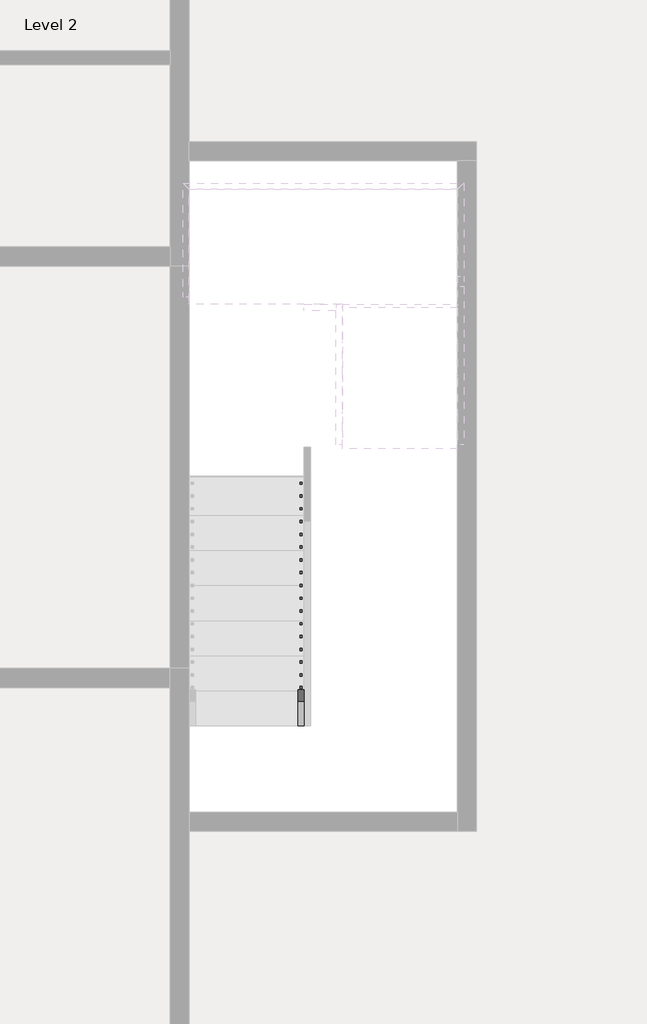
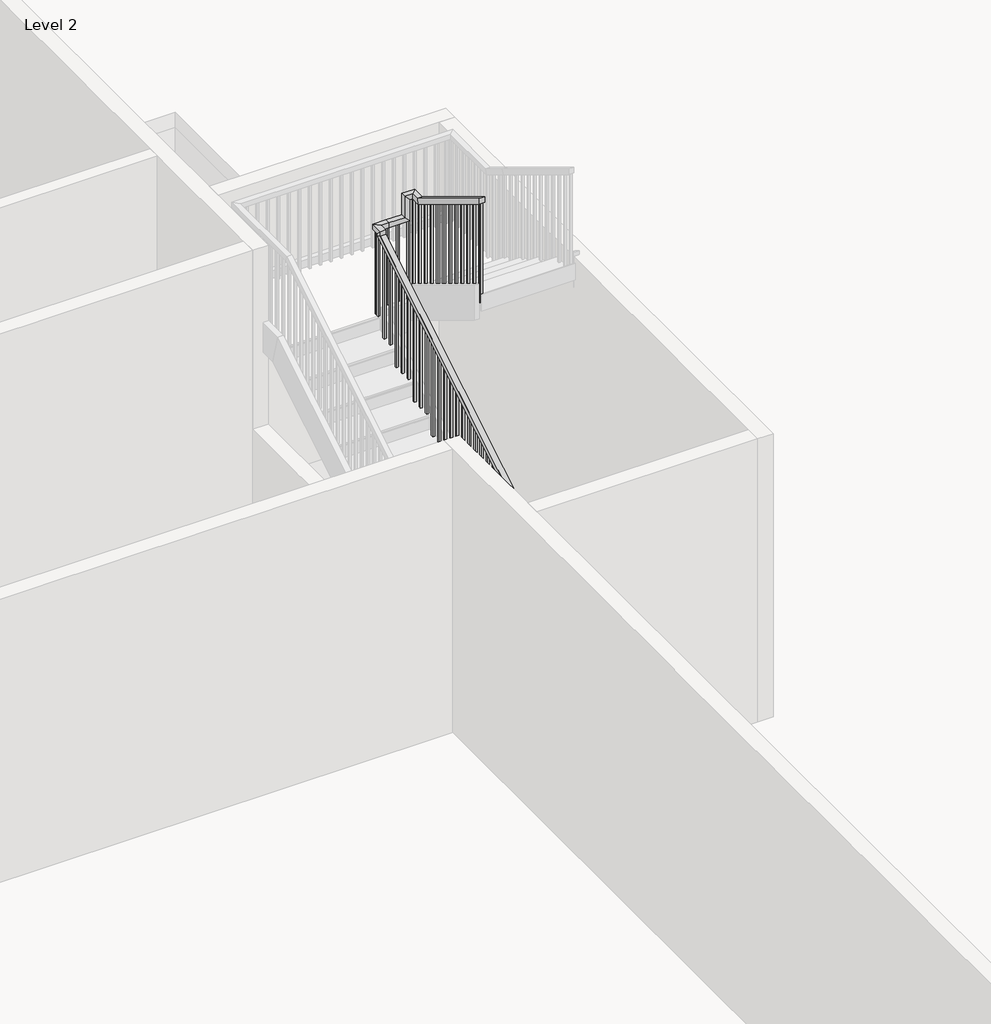
# One storey, part 7 of 8: 1 railing.
"""IFC4 building model written with IfcOpenShell, lengths in millimetres."""

from ifc_helpers import new_model, si_unit, frame, origin, place, context, project, spatial, polyline, outline, extrude, faceted_brep, element, save

model = new_model("IFC4")

# Units and contexts
model_context = context("Model", 3, world=origin())
ifc_project = project(units=[si_unit("LENGTHUNIT", "METRE", prefix="MILLI")], contexts=[model_context])

# Site, building, storey
site = spatial("IfcSite", under=ifc_project)
building = spatial("IfcBuilding", under=site)
storey = spatial("IfcBuildingStorey", under=building, Name="Level 2", Elevation=28282.6172466)

# Railing
placement = place(None, origin())
element("IfcRailing", 1, ObjectType="Handrail - Rectangular", at=placement, inside=storey, context=model_context, shape_type="SolidModel", body=[
    faceted_brep([(-2753.8415084, 19841.9216096, 29366.3505799), (-2753.8415084, 19841.9216096, 29306.9491197), (-2703.0415084, 19841.9216096, 29306.9491197), (-2703.0415084, 19841.9216096, 29366.3505799), (-2753.8415084, 23118.5216096, 31352.1687618), (-2753.8415084, 23169.3216096, 31323.5551803), (-2703.0415084, 23169.3216096, 31323.5551803), (-2703.0415084, 23118.5216096, 31352.1687618), (-2753.8415084, 23118.5216096, 31398.3505799), (-2753.8415084, 23169.3216096, 31347.5505799), (-2703.0415084, 23169.3216096, 31347.5505799), (-2703.0415084, 23118.5216096, 31398.3505799), (-2753.8415084, 23245.5216096, 31398.3505799), (-2753.8415084, 23245.5216096, 31347.5505799), (-2703.0415084, 23194.7216096, 31347.5505799), (-2703.0415084, 23194.7216096, 31398.3505799), (-2626.8415084, 23245.5216096, 31398.3505799), (-2626.8415084, 23245.5216096, 31347.5505799), (-2626.8415084, 23194.7216096, 31347.5505799), (-2626.8415084, 23194.7216096, 31398.3505799), (-2474.4415084, 23245.5216096, 31398.3505799), (-2423.6415084, 23245.5216096, 31347.5505799), (-2423.6415084, 23194.7216096, 31347.5505799), (-2474.4415084, 23194.7216096, 31398.3505799), (-2474.4415084, 23245.5216096, 31613.8657314), (-2423.6415084, 23245.5216096, 31563.0657314), (-2423.6415084, 23194.7216096, 31563.0657314), (-2474.4415084, 23194.7216096, 31613.8657314), (-2347.4415084, 23245.5216096, 31613.8657314), (-2347.4415084, 23245.5216096, 31563.0657314), (-2398.2415084, 23194.7216096, 31563.0657314), (-2398.2415084, 23194.7216096, 31613.8657314), (-2347.4415084, 23118.5216096, 31613.8657314), (-2347.4415084, 23104.3292002, 31563.0657314), (-2398.2415084, 23104.3292002, 31563.0657314), (-2398.2415084, 23118.5216096, 31613.8657314), (-2347.4415084, 22077.1216096, 32245.0172466), (-2398.2415084, 22077.1216096, 32245.0172466), (-2398.2415084, 22077.1216096, 32185.6157863), (-2347.4415084, 22077.1216096, 32185.6157863)], [[[0, 1, 2, 3]], [[1, 0, 4, 5]], [[2, 1, 5, 6]], [[3, 2, 6, 7]], [[0, 3, 7, 4]], [[5, 4, 8, 9]], [[6, 5, 9, 10]], [[7, 6, 10, 11]], [[4, 7, 11, 8]], [[9, 8, 12, 13]], [[10, 9, 13, 14]], [[11, 10, 14, 15]], [[8, 11, 15, 12]], [[13, 12, 16, 17]], [[14, 13, 17, 18]], [[15, 14, 18, 19]], [[12, 15, 19, 16]], [[17, 16, 20, 21]], [[18, 17, 21, 22]], [[19, 18, 22, 23]], [[16, 19, 23, 20]], [[21, 20, 24, 25]], [[22, 21, 25, 26]], [[23, 22, 26, 27]], [[20, 23, 27, 24]], [[25, 24, 28, 29]], [[26, 25, 29, 30]], [[27, 26, 30, 31]], [[24, 27, 31, 28]], [[29, 28, 32, 33]], [[30, 29, 33, 34]], [[31, 30, 34, 35]], [[28, 31, 35, 32]], [[36, 37, 38, 39]], [[33, 32, 36, 39]], [[34, 33, 39, 38]], [[35, 34, 38, 37]], [[32, 35, 37, 36]]]),
    extrude(outline(polyline([(22092.9966096, 32175.9945742), (22112.0466096, 32164.4491197), (22112.0466096, 31161.2839133), (22092.9966096, 31161.2839133), (22092.9966096, 32175.9945742)])), frame((-2382.3665084, 0.0, 0.0), z_axis=(1.0, 0.0, 0.0), x_axis=(0.0, 1.0, 0.0)), (0.0, 0.0, 1.0), 19.05),
    extrude(outline(polyline([(22194.5966096, 32114.4188166), (22213.6466096, 32102.8733621), (22213.6466096, 31161.2839133), (22194.5966096, 31161.2839133), (22194.5966096, 32114.4188166)])), frame((-2382.3665084, 0.0, 0.0), z_axis=(1.0, 0.0, 0.0), x_axis=(0.0, 1.0, 0.0)), (0.0, 0.0, 1.0), 19.05),
    extrude(outline(polyline([(22296.1966096, 32052.8430591), (22315.2466096, 32041.2976045), (22315.2466096, 31161.2839133), (22296.1966096, 31161.2839133), (22296.1966096, 32052.8430591)])), frame((-2382.3665084, 0.0, 0.0), z_axis=(1.0, 0.0, 0.0), x_axis=(0.0, 1.0, 0.0)), (0.0, 0.0, 1.0), 19.05),
    extrude(outline(polyline([(22397.7966096, 31991.2673015), (22416.8466096, 31979.721847), (22416.8466096, 30991.9505799), (22397.7966096, 30991.9505799), (22397.7966096, 31991.2673015)])), frame((-2382.3665084, 0.0, 0.0), z_axis=(1.0, 0.0, 0.0), x_axis=(0.0, 1.0, 0.0)), (0.0, 0.0, 1.0), 19.05),
    extrude(outline(polyline([(22499.3966096, 31929.6915439), (22518.4466096, 31918.1460894), (22518.4466096, 30991.9505799), (22499.3966096, 30991.9505799), (22499.3966096, 31929.6915439)])), frame((-2382.3665084, 0.0, 0.0), z_axis=(1.0, 0.0, 0.0), x_axis=(0.0, 1.0, 0.0)), (0.0, 0.0, 1.0), 19.05),
    extrude(outline(polyline([(22600.9966096, 31868.1157863), (22620.0466096, 31856.5703318), (22620.0466096, 30991.9505799), (22600.9966096, 30991.9505799), (22600.9966096, 31868.1157863)])), frame((-2382.3665084, 0.0, 0.0), z_axis=(1.0, 0.0, 0.0), x_axis=(0.0, 1.0, 0.0)), (0.0, 0.0, 1.0), 19.05),
    extrude(outline(polyline([(22702.5966096, 31806.5400288), (22721.6466096, 31794.9945742), (22721.6466096, 30822.6172466), (22702.5966096, 30822.6172466), (22702.5966096, 31806.5400288)])), frame((-2382.3665084, 0.0, 0.0), z_axis=(1.0, 0.0, 0.0), x_axis=(0.0, 1.0, 0.0)), (0.0, 0.0, 1.0), 19.05),
    extrude(outline(polyline([(22804.1966096, 31744.9642712), (22823.2466096, 31733.4188166), (22823.2466096, 30822.6172466), (22804.1966096, 30822.6172466), (22804.1966096, 31744.9642712)])), frame((-2382.3665084, 0.0, 0.0), z_axis=(1.0, 0.0, 0.0), x_axis=(0.0, 1.0, 0.0)), (0.0, 0.0, 1.0), 19.05),
    extrude(outline(polyline([(22905.7966096, 31683.3885136), (22924.8466096, 31671.8430591), (22924.8466096, 30822.6172466), (22905.7966096, 30822.6172466), (22905.7966096, 31683.3885136)])), frame((-2382.3665084, 0.0, 0.0), z_axis=(1.0, 0.0, 0.0), x_axis=(0.0, 1.0, 0.0)), (0.0, 0.0, 1.0), 19.05),
    extrude(outline(polyline([(23007.3966096, 31621.812756), (23026.4466096, 31610.2673015), (23026.4466096, 30653.2839133), (23007.3966096, 30653.2839133), (23007.3966096, 31621.812756)])), frame((-2382.3665084, 0.0, 0.0), z_axis=(1.0, 0.0, 0.0), x_axis=(0.0, 1.0, 0.0)), (0.0, 0.0, 1.0), 19.05),
    extrude(outline(polyline([(23108.9966096, 31560.2369985), (23128.0466096, 31548.6915439), (23128.0466096, 30653.2839133), (23108.9966096, 30653.2839133), (23108.9966096, 31560.2369985)])), frame((-2382.3665084, 0.0, 0.0), z_axis=(1.0, 0.0, 0.0), x_axis=(0.0, 1.0, 0.0)), (0.0, 0.0, 1.0), 19.05),
    extrude(outline(polyline([(-2433.1665084, 23210.5966096), (-2433.1665084, 23229.6466096), (-2414.1165084, 23229.6466096), (-2414.1165084, 23210.5966096), (-2433.1665084, 23210.5966096)])), frame((0.0, 0.0, 30483.9505799), z_axis=(0.0, 0.0, 1.0), x_axis=(1.0, 0.0, 0.0)), (0.0, 0.0, 1.0), 1079.1151515),
    extrude(outline(polyline([(-2534.7665084, 23210.5966096), (-2534.7665084, 23229.6466096), (-2515.7165084, 23229.6466096), (-2515.7165084, 23210.5966096), (-2534.7665084, 23210.5966096)])), frame((0.0, 0.0, 30483.9505799), z_axis=(0.0, 0.0, 1.0), x_axis=(1.0, 0.0, 0.0)), (0.0, 0.0, 1.0), 863.6),
    extrude(outline(polyline([(-2636.3665084, 23210.5966096), (-2636.3665084, 23229.6466096), (-2617.3165084, 23229.6466096), (-2617.3165084, 23210.5966096), (-2636.3665084, 23210.5966096)])), frame((0.0, 0.0, 30483.9505799), z_axis=(0.0, 0.0, 1.0), x_axis=(1.0, 0.0, 0.0)), (0.0, 0.0, 1.0), 863.6),
    extrude(outline(polyline([(-2718.9165084, 23185.1966096), (-2737.9665084, 23185.1966096), (-2737.9665084, 23204.2466096), (-2718.9165084, 23204.2466096), (-2718.9165084, 23185.1966096)])), frame((0.0, 0.0, 30483.9505799), z_axis=(0.0, 0.0, 1.0), x_axis=(1.0, 0.0, 0.0)), (0.0, 0.0, 1.0), 863.6),
    extrude(outline(polyline([(23083.5966096, 31271.6006348), (23102.6466096, 31283.1460894), (23102.6466096, 30314.6172466), (23083.5966096, 30314.6172466), (23083.5966096, 31271.6006348)])), frame((-2737.9665084, 0.0, 0.0), z_axis=(1.0, 0.0, 0.0), x_axis=(0.0, 1.0, 0.0)), (0.0, 0.0, 1.0), 19.05),
    extrude(outline(polyline([(22981.9966096, 31210.0248773), (23001.0466096, 31221.5703318), (23001.0466096, 30314.6172466), (22981.9966096, 30314.6172466), (22981.9966096, 31210.0248773)])), frame((-2737.9665084, 0.0, 0.0), z_axis=(1.0, 0.0, 0.0), x_axis=(0.0, 1.0, 0.0)), (0.0, 0.0, 1.0), 19.05),
    extrude(outline(polyline([(22880.3966096, 31148.4491197), (22899.4466096, 31159.9945742), (22899.4466096, 30145.2839133), (22880.3966096, 30145.2839133), (22880.3966096, 31148.4491197)])), frame((-2737.9665084, 0.0, 0.0), z_axis=(1.0, 0.0, 0.0), x_axis=(0.0, 1.0, 0.0)), (0.0, 0.0, 1.0), 19.05),
    extrude(outline(polyline([(22778.7966096, 31086.8733621), (22797.8466096, 31098.4188167), (22797.8466096, 30145.2839133), (22778.7966096, 30145.2839133), (22778.7966096, 31086.8733621)])), frame((-2737.9665084, 0.0, 0.0), z_axis=(1.0, 0.0, 0.0), x_axis=(0.0, 1.0, 0.0)), (0.0, 0.0, 1.0), 19.05),
    extrude(outline(polyline([(22677.1966096, 31025.2976045), (22696.2466096, 31036.8430591), (22696.2466096, 30145.2839133), (22677.1966096, 30145.2839133), (22677.1966096, 31025.2976045)])), frame((-2737.9665084, 0.0, 0.0), z_axis=(1.0, 0.0, 0.0), x_axis=(0.0, 1.0, 0.0)), (0.0, 0.0, 1.0), 19.05),
    extrude(outline(polyline([(22575.5966096, 30963.721847), (22594.6466096, 30975.2673015), (22594.6466096, 29975.9505799), (22575.5966096, 29975.9505799), (22575.5966096, 30963.721847)])), frame((-2737.9665084, 0.0, 0.0), z_axis=(1.0, 0.0, 0.0), x_axis=(0.0, 1.0, 0.0)), (0.0, 0.0, 1.0), 19.05),
    extrude(outline(polyline([(22473.9966096, 30902.1460894), (22493.0466096, 30913.6915439), (22493.0466096, 29975.9505799), (22473.9966096, 29975.9505799), (22473.9966096, 30902.1460894)])), frame((-2737.9665084, 0.0, 0.0), z_axis=(1.0, 0.0, 0.0), x_axis=(0.0, 1.0, 0.0)), (0.0, 0.0, 1.0), 19.05),
    extrude(outline(polyline([(22372.3966096, 30840.5703318), (22391.4466096, 30852.1157863), (22391.4466096, 29975.9505799), (22372.3966096, 29975.9505799), (22372.3966096, 30840.5703318)])), frame((-2737.9665084, 0.0, 0.0), z_axis=(1.0, 0.0, 0.0), x_axis=(0.0, 1.0, 0.0)), (0.0, 0.0, 1.0), 19.05),
    extrude(outline(polyline([(22270.7966096, 30778.9945742), (22289.8466096, 30790.5400288), (22289.8466096, 29806.6172466), (22270.7966096, 29806.6172466), (22270.7966096, 30778.9945742)])), frame((-2737.9665084, 0.0, 0.0), z_axis=(1.0, 0.0, 0.0), x_axis=(0.0, 1.0, 0.0)), (0.0, 0.0, 1.0), 19.05),
    extrude(outline(polyline([(22169.1966096, 30717.4188167), (22188.2466096, 30728.9642712), (22188.2466096, 29806.6172466), (22169.1966096, 29806.6172466), (22169.1966096, 30717.4188167)])), frame((-2737.9665084, 0.0, 0.0), z_axis=(1.0, 0.0, 0.0), x_axis=(0.0, 1.0, 0.0)), (0.0, 0.0, 1.0), 19.05),
    extrude(outline(polyline([(22067.5966096, 30655.8430591), (22086.6466096, 30667.3885136), (22086.6466096, 29806.6172466), (22067.5966096, 29806.6172466), (22067.5966096, 30655.8430591)])), frame((-2737.9665084, 0.0, 0.0), z_axis=(1.0, 0.0, 0.0), x_axis=(0.0, 1.0, 0.0)), (0.0, 0.0, 1.0), 19.05),
    extrude(outline(polyline([(21965.9966096, 30594.2673015), (21985.0466096, 30605.812756), (21985.0466096, 29637.2839133), (21965.9966096, 29637.2839133), (21965.9966096, 30594.2673015)])), frame((-2737.9665084, 0.0, 0.0), z_axis=(1.0, 0.0, 0.0), x_axis=(0.0, 1.0, 0.0)), (0.0, 0.0, 1.0), 19.05),
    extrude(outline(polyline([(21864.3966096, 30532.6915439), (21883.4466096, 30544.2369985), (21883.4466096, 29637.2839133), (21864.3966096, 29637.2839133), (21864.3966096, 30532.6915439)])), frame((-2737.9665084, 0.0, 0.0), z_axis=(1.0, 0.0, 0.0), x_axis=(0.0, 1.0, 0.0)), (0.0, 0.0, 1.0), 19.05),
    extrude(outline(polyline([(21762.7966096, 30471.1157863), (21781.8466096, 30482.6612409), (21781.8466096, 29467.9505799), (21762.7966096, 29467.9505799), (21762.7966096, 30471.1157863)])), frame((-2737.9665084, 0.0, 0.0), z_axis=(1.0, 0.0, 0.0), x_axis=(0.0, 1.0, 0.0)), (0.0, 0.0, 1.0), 19.05),
    extrude(outline(polyline([(21661.1966096, 30409.5400288), (21680.2466096, 30421.0854833), (21680.2466096, 29467.9505799), (21661.1966096, 29467.9505799), (21661.1966096, 30409.5400288)])), frame((-2737.9665084, 0.0, 0.0), z_axis=(1.0, 0.0, 0.0), x_axis=(0.0, 1.0, 0.0)), (0.0, 0.0, 1.0), 19.05),
    extrude(outline(polyline([(21559.5966096, 30347.9642712), (21578.6466096, 30359.5097257), (21578.6466096, 29467.9505799), (21559.5966096, 29467.9505799), (21559.5966096, 30347.9642712)])), frame((-2737.9665084, 0.0, 0.0), z_axis=(1.0, 0.0, 0.0), x_axis=(0.0, 1.0, 0.0)), (0.0, 0.0, 1.0), 19.05),
    extrude(outline(polyline([(21457.9966096, 30286.3885136), (21477.0466096, 30297.9339682), (21477.0466096, 29298.6172466), (21457.9966096, 29298.6172466), (21457.9966096, 30286.3885136)])), frame((-2737.9665084, 0.0, 0.0), z_axis=(1.0, 0.0, 0.0), x_axis=(0.0, 1.0, 0.0)), (0.0, 0.0, 1.0), 19.05),
    extrude(outline(polyline([(21356.3966096, 30224.812756), (21375.4466096, 30236.3582106), (21375.4466096, 29298.6172466), (21356.3966096, 29298.6172466), (21356.3966096, 30224.812756)])), frame((-2737.9665084, 0.0, 0.0), z_axis=(1.0, 0.0, 0.0), x_axis=(0.0, 1.0, 0.0)), (0.0, 0.0, 1.0), 19.05),
    extrude(outline(polyline([(21254.7966096, 30163.2369985), (21273.8466096, 30174.782453), (21273.8466096, 29298.6172466), (21254.7966096, 29298.6172466), (21254.7966096, 30163.2369985)])), frame((-2737.9665084, 0.0, 0.0), z_axis=(1.0, 0.0, 0.0), x_axis=(0.0, 1.0, 0.0)), (0.0, 0.0, 1.0), 19.05),
    extrude(outline(polyline([(21153.1966096, 30101.6612409), (21172.2466096, 30113.2066954), (21172.2466096, 29129.2839133), (21153.1966096, 29129.2839133), (21153.1966096, 30101.6612409)])), frame((-2737.9665084, 0.0, 0.0), z_axis=(1.0, 0.0, 0.0), x_axis=(0.0, 1.0, 0.0)), (0.0, 0.0, 1.0), 19.05),
    extrude(outline(polyline([(21051.5966096, 30040.0854833), (21070.6466096, 30051.6309379), (21070.6466096, 29129.2839133), (21051.5966096, 29129.2839133), (21051.5966096, 30040.0854833)])), frame((-2737.9665084, 0.0, 0.0), z_axis=(1.0, 0.0, 0.0), x_axis=(0.0, 1.0, 0.0)), (0.0, 0.0, 1.0), 19.05),
    extrude(outline(polyline([(20949.9966096, 29978.5097257), (20969.0466096, 29990.0551803), (20969.0466096, 29129.2839133), (20949.9966096, 29129.2839133), (20949.9966096, 29978.5097257)])), frame((-2737.9665084, 0.0, 0.0), z_axis=(1.0, 0.0, 0.0), x_axis=(0.0, 1.0, 0.0)), (0.0, 0.0, 1.0), 19.05),
    extrude(outline(polyline([(20848.3966096, 29916.9339682), (20867.4466096, 29928.4794227), (20867.4466096, 28959.9505799), (20848.3966096, 28959.9505799), (20848.3966096, 29916.9339682)])), frame((-2737.9665084, 0.0, 0.0), z_axis=(1.0, 0.0, 0.0), x_axis=(0.0, 1.0, 0.0)), (0.0, 0.0, 1.0), 19.05),
    extrude(outline(polyline([(20746.7966096, 29855.3582106), (20765.8466096, 29866.9036651), (20765.8466096, 28959.9505799), (20746.7966096, 28959.9505799), (20746.7966096, 29855.3582106)])), frame((-2737.9665084, 0.0, 0.0), z_axis=(1.0, 0.0, 0.0), x_axis=(0.0, 1.0, 0.0)), (0.0, 0.0, 1.0), 19.05),
    extrude(outline(polyline([(20645.1966096, 29793.782453), (20664.2466096, 29805.3279076), (20664.2466096, 28790.6172466), (20645.1966096, 28790.6172466), (20645.1966096, 29793.782453)])), frame((-2737.9665084, 0.0, 0.0), z_axis=(1.0, 0.0, 0.0), x_axis=(0.0, 1.0, 0.0)), (0.0, 0.0, 1.0), 19.05),
    extrude(outline(polyline([(20543.5966096, 29732.2066954), (20562.6466096, 29743.75215), (20562.6466096, 28790.6172466), (20543.5966096, 28790.6172466), (20543.5966096, 29732.2066954)])), frame((-2737.9665084, 0.0, 0.0), z_axis=(1.0, 0.0, 0.0), x_axis=(0.0, 1.0, 0.0)), (0.0, 0.0, 1.0), 19.05),
    extrude(outline(polyline([(20441.9966096, 29670.6309379), (20461.0466096, 29682.1763924), (20461.0466096, 28790.6172466), (20441.9966096, 28790.6172466), (20441.9966096, 29670.6309379)])), frame((-2737.9665084, 0.0, 0.0), z_axis=(1.0, 0.0, 0.0), x_axis=(0.0, 1.0, 0.0)), (0.0, 0.0, 1.0), 19.05),
    extrude(outline(polyline([(20340.3966096, 29609.0551803), (20359.4466096, 29620.6006348), (20359.4466096, 28621.2839133), (20340.3966096, 28621.2839133), (20340.3966096, 29609.0551803)])), frame((-2737.9665084, 0.0, 0.0), z_axis=(1.0, 0.0, 0.0), x_axis=(0.0, 1.0, 0.0)), (0.0, 0.0, 1.0), 19.05),
    extrude(outline(polyline([(20238.7966096, 29547.4794227), (20257.8466096, 29559.0248773), (20257.8466096, 28621.2839133), (20238.7966096, 28621.2839133), (20238.7966096, 29547.4794227)])), frame((-2737.9665084, 0.0, 0.0), z_axis=(1.0, 0.0, 0.0), x_axis=(0.0, 1.0, 0.0)), (0.0, 0.0, 1.0), 19.05),
    extrude(outline(polyline([(20137.1966096, 29485.9036651), (20156.2466096, 29497.4491197), (20156.2466096, 28621.2839133), (20137.1966096, 28621.2839133), (20137.1966096, 29485.9036651)])), frame((-2737.9665084, 0.0, 0.0), z_axis=(1.0, 0.0, 0.0), x_axis=(0.0, 1.0, 0.0)), (0.0, 0.0, 1.0), 19.05),
    extrude(outline(polyline([(20035.5966096, 29424.3279076), (20054.6466096, 29435.8733621), (20054.6466096, 28451.9505799), (20035.5966096, 28451.9505799), (20035.5966096, 29424.3279076)])), frame((-2737.9665084, 0.0, 0.0), z_axis=(1.0, 0.0, 0.0), x_axis=(0.0, 1.0, 0.0)), (0.0, 0.0, 1.0), 19.05),
    extrude(outline(polyline([(19933.9966096, 29362.75215), (19953.0466096, 29374.2976045), (19953.0466096, 28451.9505799), (19933.9966096, 28451.9505799), (19933.9966096, 29362.75215)])), frame((-2737.9665084, 0.0, 0.0), z_axis=(1.0, 0.0, 0.0), x_axis=(0.0, 1.0, 0.0)), (0.0, 0.0, 1.0), 19.05),
    extrude(outline(polyline([(-2382.3665084, 23210.5966096), (-2382.3665084, 23229.6466096), (-2363.3165084, 23229.6466096), (-2363.3165084, 23210.5966096), (-2382.3665084, 23210.5966096)])), frame((0.0, 0.0, 30483.9505799), z_axis=(0.0, 0.0, 1.0), x_axis=(1.0, 0.0, 0.0)), (0.0, 0.0, 1.0), 1079.1151515),
    extrude(outline(polyline([(-2718.9165084, 23210.5966096), (-2737.9665084, 23210.5966096), (-2737.9665084, 23229.6466096), (-2718.9165084, 23229.6466096), (-2718.9165084, 23210.5966096)])), frame((0.0, 0.0, 30483.9505799), z_axis=(0.0, 0.0, 1.0), x_axis=(1.0, 0.0, 0.0)), (0.0, 0.0, 1.0), 863.6),
    extrude(outline(polyline([(22077.1216096, 32185.6157863), (22096.1716096, 32174.0703318), (22096.1716096, 31161.2839133), (22077.1216096, 31161.2839133), (22077.1216096, 32185.6157863)])), frame((-2382.3665084, 0.0, 0.0), z_axis=(1.0, 0.0, 0.0), x_axis=(0.0, 1.0, 0.0)), (0.0, 0.0, 1.0), 19.05),
    extrude(outline(polyline([(19841.9216096, 29306.9491197), (19860.9716096, 29318.4945742), (19860.9716096, 28451.9505799), (19841.9216096, 28451.9505799), (19841.9216096, 29306.9491197)])), frame((-2737.9665084, 0.0, 0.0), z_axis=(1.0, 0.0, 0.0), x_axis=(0.0, 1.0, 0.0)), (0.0, 0.0, 1.0), 19.05),
])

save(model, "model.ifc")

# Revit data of these elements
# Type "Handrail - Rectangular"
#   Assembly Code = "C2010400"
#   built-in parameter 1008612 = 0.0416667 (stored number, unit not read)
#   built-in parameter 1008611 = 0.0416667 (stored number, unit not read)
#   built-in parameter 1008609 = 0.333333 (stored number, unit not read)
#   built-in parameter 1008604 = 0.166667 (stored number, unit not read)
#   built-in parameter 1008603 = 0.166667 (stored number, unit not read)
#   Railing Height = 3' - 0"
#   built-in parameter 1008630 = 2
#   built-in parameter 1008610 = 2
#   built-in parameter 1008618 = Baluster - Square : 3/4"
# Element 1 (IfcRailing, "Handrail - Rectangular")
#   Phase Created = New Construction
